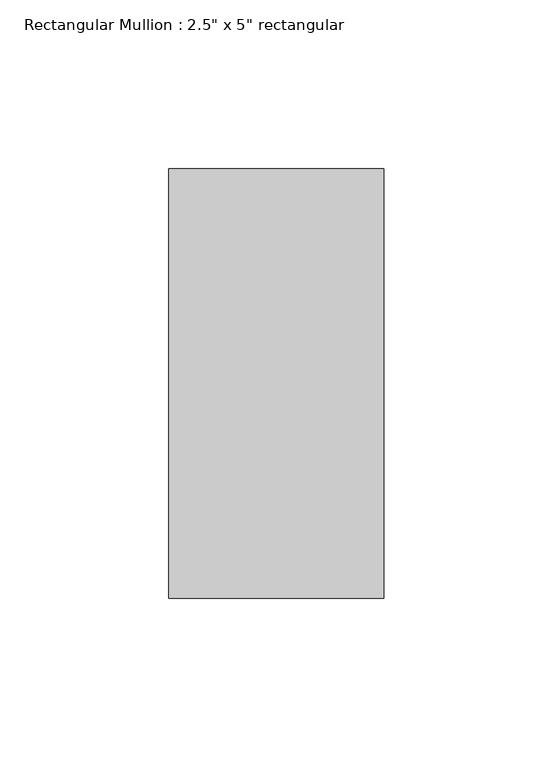
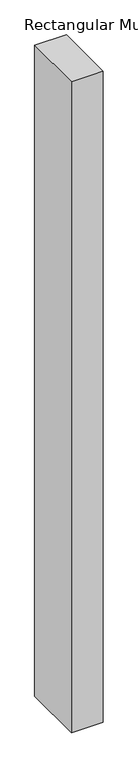
"""IFC4 building model written with IfcOpenShell, lengths in millimetres: member geometry."""

from ifc_helpers import new_model, si_unit, frame, origin, place, context, project, spatial, polyline, outline, extrude, source, transform, mapped, element, save


def member_4214a330(model_context):
    return source(origin(), model_context, "Body", "SweptSolid", [
        extrude(outline(polyline([(0.0, 63.5), (0.0, -63.5), (-63.5, -63.5), (-63.5, 63.5), (0.0, 63.5)])), frame((0.0, 0.0, -1375.9446538), z_axis=(0.0, 0.0, 1.0), x_axis=(1.0, 0.0, 0.0)), (0.0, 0.0, 1.0), 1375.9446538),
    ])


if __name__ == "__main__":
    model = new_model("IFC4")
    model_context = context("Model", 3, world=origin())
    ifc_project = project(units=[si_unit("LENGTHUNIT", "METRE", prefix="MILLI")], contexts=[model_context])
    site = spatial("IfcSite", under=ifc_project)
    building = spatial("IfcBuilding", under=site)
    placement = place(None, origin())
    member_shape = member_4214a330(model_context)
    element("IfcMember", 1, ObjectType="Rectangular Mullion : 2.5\" x 5\" rectangular", at=placement, inside=building, context=model_context, shape_type="MappedRepresentation", body=[
        mapped(member_shape, transform((0.0, 0.0, 0.0), x_axis=(1.0, 0.0, 0.0), y_axis=(0.0, 1.0, 0.0), z_axis=(0.0, 0.0, 1.0))),
    ])
    save(model, "model.ifc")

# Revit data of these elements
# Type "Rectangular Mullion : 2.5\" x 5\" rectangular"
#   built-in parameter 1007304 = 0.416667 (stored number, unit not read)
#   built-in parameter 1007301 = 0.104167 (stored number, unit not read)
#   built-in parameter 1007300 = 0.104167 (stored number, unit not read)
# Element 1 (IfcMember, "Rectangular Mullion : 2.5\" x 5\" rectangular")
#   Materials on its faces: "Aluminum"
# Materials
#   "Aluminum": class "Metal", colour RGB 247 247 247, transparency 0, Description = "Aluminum 6061", Cost = 0
